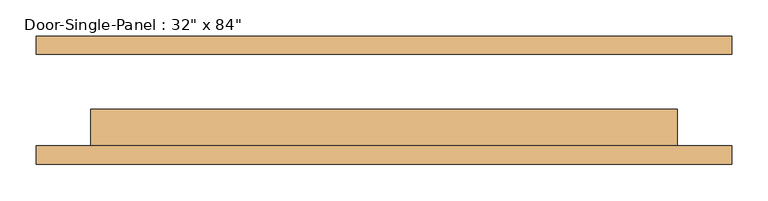
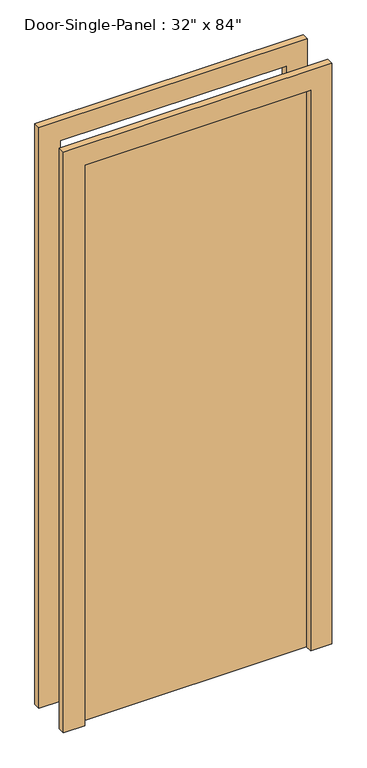
"""IFC4 building model written with IfcOpenShell, lengths in millimetres: door geometry."""

from ifc_helpers import new_model, si_unit, frame, origin, origin_with_axes, place, context, project, spatial, polyline, outline, extrude, source, transform, mapped, element, save


def door_af63d1be(model_context):
    return source(origin(), model_context, "Body", "SweptSolid", [
        extrude(outline(polyline([(406.4, -12.7), (406.4, -63.5), (-406.4, -63.5), (-406.4, -12.7), (406.4, -12.7)])), origin_with_axes(), (0.0, 0.0, 1.0), 2133.6),
        extrude(outline(polyline([(2209.8, -482.6), (0.0, -482.6), (0.0, -406.4), (2133.6, -406.4), (2133.6, 406.4), (0.0, 406.4), (0.0, 482.6), (2209.8, 482.6), (2209.8, -482.6)])), frame((0.0, -88.9, 0.0), z_axis=(0.0, 1.0, 0.0), x_axis=(0.0, 0.0, 1.0)), (0.0, 0.0, 1.0), 25.4),
        extrude(outline(polyline([(2209.8, 482.6), (2209.8, -482.6), (0.0, -482.6), (0.0, -406.4), (2133.6, -406.4), (2133.6, 406.4), (0.0, 406.4), (0.0, 482.6), (2209.8, 482.6)])), frame((0.0, 63.5, 0.0), z_axis=(0.0, 1.0, 0.0), x_axis=(0.0, 0.0, 1.0)), (0.0, 0.0, 1.0), 25.4),
    ])


if __name__ == "__main__":
    model = new_model("IFC4")
    model_context = context("Model", 3, world=origin())
    ifc_project = project(units=[si_unit("LENGTHUNIT", "METRE", prefix="MILLI")], contexts=[model_context])
    site = spatial("IfcSite", under=ifc_project)
    building = spatial("IfcBuilding", under=site)
    placement = place(None, origin())
    door_shape = door_af63d1be(model_context)
    element("IfcDoor", 1, ObjectType="Door-Single-Panel : 32\" x 84\"", at=placement, inside=building, context=model_context, shape_type="MappedRepresentation", body=[
        mapped(door_shape, transform((0.0, 0.0, 0.0), x_axis=(1.0, 0.0, 0.0), y_axis=(0.0, 1.0, 0.0), z_axis=(0.0, 0.0, 1.0))),
    ])
    save(model, "model.ifc")

# Revit data of these elements
# Type "Door-Single-Panel : 32\" x 84\""
#   Type Mark = "11"
#   Construction Type Id = "DOOR"
#   Assembly Code = "C1020300"
#   Analytic Construction = "Wooden"
#   Thickness = 0' - 2"
#   Thermal Resistance (R) = 2.5876 (h·ft²·°F)/BTU
#   Swing Angle [instance default] = 90.00°
#   Heat Transfer Coefficient (U) = 0.3865 BTU/(h·ft²·°F)
#   Height = 7' - 0"
#   Trim Projection Ext = 0' - 1"
#   Trim Projection Int = 0' - 1"
#   Trim Width = 0' - 3"
#   Width = 2' - 8"
#   Define Thermal Properties by = 1
#   Panel Material = Wood - Birch - Solid Stained Light Low Gloss
#   Trim Material = Paint - Sienna
#   Visual Light Transmittance = 0
#   Solar Heat Gain Coefficient = 0
#   Function = (empty or 0)
#   Wall Closure = (empty or 0)
# Element 1 (IfcDoor, "Door-Single-Panel : 32\" x 84\"")
#   Materials on its faces: "Paint - Sienna", "Wood - Birch - Solid Stained Light Low Gloss"
# Materials
#   "Wood - Birch - Solid Stained Light Low Gloss": class "Wood", colour RGB 210 159 95, transparency 0, Cost = 0
#   "Paint - Sienna": colour RGB 118 70 51, transparency 0, Cost = 0
